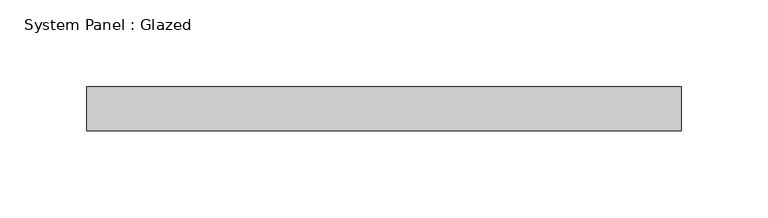
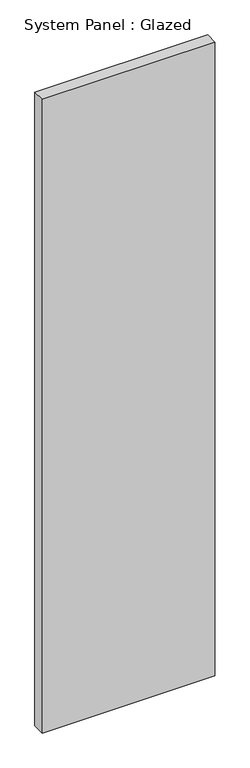
"""IFC4 building model written with IfcOpenShell, lengths in millimetres: plate geometry, System Panel : Glazed."""

from ifc_helpers import new_model, si_unit, origin, origin_with_axes, place, context, project, spatial, polyline, outline, extrude, source, transform, mapped, element, save


def system_panel_glazed_4bf0fdf0(model_context):
    return source(origin(), model_context, "Body", "SweptSolid", [
        extrude(outline(polyline([(171.45, 19.05), (-171.45, 19.05), (-171.45, 44.45), (171.45, 44.45), (171.45, 19.05)])), origin_with_axes(), (0.0, 0.0, 1.0), 1330.1797686),
    ])


if __name__ == "__main__":
    model = new_model("IFC4")
    model_context = context("Model", 3, world=origin())
    ifc_project = project(units=[si_unit("LENGTHUNIT", "METRE", prefix="MILLI")], contexts=[model_context])
    site = spatial("IfcSite", under=ifc_project)
    building = spatial("IfcBuilding", under=site)
    placement = place(None, origin())
    system_panel_glazed_shape = system_panel_glazed_4bf0fdf0(model_context)
    element("IfcPlate", 1, ObjectType="System Panel : Glazed", at=placement, inside=building, context=model_context, shape_type="MappedRepresentation", body=[
        mapped(system_panel_glazed_shape, transform((0.0, 0.0, 0.0), x_axis=(1.0, 0.0, 0.0), y_axis=(0.0, 1.0, 0.0), z_axis=(0.0, 0.0, 1.0))),
    ])
    save(model, "model.ifc")

# Revit data of these elements
# Type "System Panel : Glazed"
#   Construction Type Id = "GSP4R"
#   Analytic Construction = "1/8 in Pilkington single glazing"
#   Visual Light Transmittance = 0.9
#   Solar Heat Gain Coefficient = 0.86
#   Heat Transfer Coefficient (U) = 1.18115 BTU/(h·ft²·°F)
#   Define Thermal Properties by = 1
# Element 1 (IfcPlate, "System Panel : Glazed")
#   Materials on its faces: "Glass"
# Materials
#   "Glass": class "Glass", colour RGB 0 128 192, transparency 0.75, Description = "Soda Lime Glass", Cost = 0
